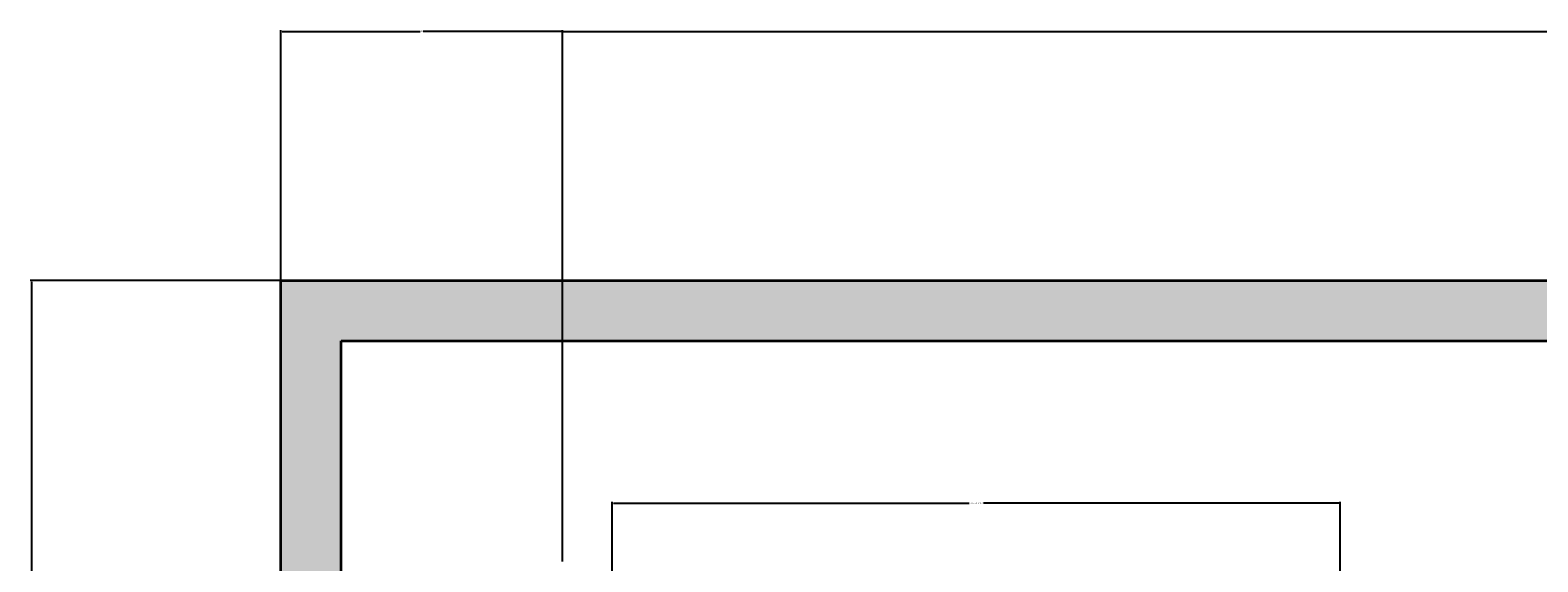
# Model space of a CAD drawing. Units: inches. Extents: x 2701 to 6846, y 811 to 2447.
# Tile 12 of 20: x 2701 to 2926, y 1462 to 1541. Entities that reach past the tile are written whole.
import ezdxf

# ---------------------------------------------------------------- set-up
doc = ezdxf.new("R2010")
doc.units = ezdxf.units.IN
doc.layers.add('A-ANNO-DIMS', color=2, linetype='Continuous', lineweight=18)
doc.layers.add('C-PROP', color=7, linetype='Continuous', lineweight=35)
doc.layers.add('C-PROP-PATT', color=18, linetype='Continuous', lineweight=13, true_color=0x000000)
doc.styles.get("Standard").update_dxf_attribs({"font": 'arial.ttf'})
doc.dimstyles.get("Standard").update_dxf_attribs({"dimtxt": 0.18, "dimasz": 0.18, "dimexe": 0.18, "dimexo": 0.0625, "dimgap": 0.09, "dimtad": 0, "dimtih": 1, "dimtoh": 1, "dimdec": 4, "dimzin": 0, "dimdsep": 46, "dimtxsty": 'Standard', "dimcen": 0.09, "dimadec": 0, "dimazin": 0, "dimtfac": 1, "dimtdec": 4, "dimtofl": 0, "dimtmove": 0, "dimatfit": 3, "dimfxl": 1, "dimtolj": 1, "dimtzin": 0, "dimarcsym": 0})

# ---------------------------------------------------------------- blocks, each defined once
blk = doc.blocks.new('*D49')
at = {"layer": 'A-ANNO-DIMS', "color": 0, "lineweight": -2, "transparency": 16777216}
for p, q in [((2787.42, 1454.59), (2787.42, 1471)), ((2787.6, 1470.82), (2840.65, 1470.82)), ((2895.86, 1470.82), (2842.8, 1470.82)), ((2896.04, 1454.59), (2896.04, 1471))]:
    blk.add_line(p, q, dxfattribs=at)
at = {"layer": 'A-ANNO-DIMS', "color": 0, "transparency": 16777216}
for points in [[(2787.6, 1470.85), (2787.6, 1470.79), (2787.42, 1470.82)], [(2895.86, 1470.85), (2895.86, 1470.79), (2896.04, 1470.82)]]:
    blk.add_solid(points, dxfattribs=at)
at = {"layer": 'Defpoints', "color": 0, "transparency": 16777216}
for p in [(2787.42, 1470.82), (2787.42, 1454.53), (2896.04, 1454.53)]:
    blk.add_point(p, dxfattribs=at)
at = {"layer": 'A-ANNO-DIMS', "color": 0, "transparency": 16777216, "insert": (2841.73, 1470.82), "char_height": 0.18, "attachment_point": 5}
blk.add_mtext('\\A1;BED GROUP 109', dxfattribs=at)
blk = doc.blocks.new('*D66')
at = {"layer": 'A-ANNO-DIMS', "color": 0, "lineweight": -2, "transparency": 16777216}
for p, q in [((2737.91, 1504.05), (2700.59, 1504.05)), ((2700.77, 1503.87), (2700.77, 1180.23)), ((2700.77, 856.23), (2700.77, 1179.87)), ((2737.91, 856.05), (2700.59, 856.05))]:
    blk.add_line(p, q, dxfattribs=at)
at = {"layer": 'A-ANNO-DIMS', "color": 0, "transparency": 16777216}
for points in [[(2700.74, 1503.87), (2700.8, 1503.87), (2700.77, 1504.05)], [(2700.74, 856.23), (2700.8, 856.23), (2700.77, 856.05)]]:
    blk.add_solid(points, dxfattribs=at)
at = {"layer": 'Defpoints', "color": 0, "transparency": 16777216}
for p in [(2700.77, 1504.05), (2737.97, 1504.05), (2737.97, 856.05)]:
    blk.add_point(p, dxfattribs=at)
at = {"layer": 'A-ANNO-DIMS', "color": 0, "transparency": 16777216, "insert": (2700.77, 1180.05), "char_height": 0.18, "attachment_point": 5}
blk.add_mtext('\\A1;648', dxfattribs=at)
blk = doc.blocks.new('*D67')
at = {"layer": 'A-ANNO-DIMS', "color": 0, "lineweight": -2, "transparency": 16777216}
for p, q in [((2779.97, 1462.11), (2779.97, 1541.43)), ((2780.15, 1541.25), (2935.68, 1541.25)), ((3091.79, 1541.25), (2936.26, 1541.25)), ((3091.97, 1462.11), (3091.97, 1541.43))]:
    blk.add_line(p, q, dxfattribs=at)
at = {"layer": 'A-ANNO-DIMS', "color": 0, "transparency": 16777216}
for points in [[(2780.15, 1541.28), (2780.15, 1541.22), (2779.97, 1541.25)], [(3091.79, 1541.28), (3091.79, 1541.22), (3091.97, 1541.25)]]:
    blk.add_solid(points, dxfattribs=at)
at = {"layer": 'Defpoints', "color": 0, "transparency": 16777216}
for p in [(3091.97, 1541.25), (2779.97, 1462.05), (3091.97, 1462.05)]:
    blk.add_point(p, dxfattribs=at)
at = {"layer": 'A-ANNO-DIMS', "color": 0, "transparency": 16777216, "insert": (2935.97, 1541.25), "char_height": 0.18, "attachment_point": 5}
blk.add_mtext('\\A1;312', dxfattribs=at)
blk = doc.blocks.new('*D69')
at = {"layer": 'A-ANNO-DIMS', "color": 0, "lineweight": -2, "transparency": 16777216}
for p, q in [((2737.97, 1504.11), (2737.97, 1541.43)), ((2738.15, 1541.25), (2758.75, 1541.25)), ((2779.79, 1541.25), (2759.19, 1541.25)), ((2779.97, 1462.11), (2779.97, 1541.43))]:
    blk.add_line(p, q, dxfattribs=at)
at = {"layer": 'A-ANNO-DIMS', "color": 0, "transparency": 16777216}
for points in [[(2738.15, 1541.28), (2738.15, 1541.22), (2737.97, 1541.25)], [(2779.79, 1541.28), (2779.79, 1541.22), (2779.97, 1541.25)]]:
    blk.add_solid(points, dxfattribs=at)
at = {"layer": 'Defpoints', "color": 0, "transparency": 16777216}
for p in [(2779.97, 1541.25), (2737.97, 1504.05), (2779.97, 1462.05)]:
    blk.add_point(p, dxfattribs=at)
at = {"layer": 'A-ANNO-DIMS', "color": 0, "transparency": 16777216, "insert": (2758.97, 1541.25), "char_height": 0.18, "attachment_point": 5}
blk.add_mtext('\\A1;42', dxfattribs=at)

msp = doc.modelspace()

# ---------------------------------------------------------------- hatches: boundary and pattern name
at = {"layer": 'C-PROP-PATT'}
h = msp.add_hatch(color=256, dxfattribs=at)
h.dxf.hatch_style = 1
h.paths.add_polyline_path([(3145.97, 1504.05), (2737.97, 1504.05), (2737.97, 967.05), (2746.97, 967.05), (2746.97, 1495.05), (3136.97, 1495.05), (3136.97, 865.05), (3130.97, 865.05), (3130.97, 856.05), (3145.97, 856.05)])
h.paths.add_polyline_path([(3070.97, 865.05), (2746.97, 865.05), (2746.97, 871.05), (2737.97, 871.05), (2737.97, 856.05), (3070.97, 856.05)], flags=17)

# ---------------------------------------------------------------- linework, layer by layer
at = {"layer": 'C-PROP'}
for p, q in [((2737.97, 1504.05), (3145.97, 1504.05)), ((2737.97, 919.05), (2737.97, 1504.05)), ((2746.97, 1495.05), (3136.97, 1495.05)), ((2746.97, 967.05), (2746.97, 1495.05))]:
    msp.add_line(p, q, dxfattribs=at)

# ---------------------------------------------------------------- dimensions: what is measured, and where the dimension line sits
at = {"layer": 'A-ANNO-DIMS'}
for base, p1, p2, picture, middle in [((2779.97, 1541.25), (2737.97, 1504.05), (2779.97, 1462.05), '*D69', (2758.97, 1541.25)), ((3091.97, 1541.25), (2779.97, 1462.05), (3091.97, 1462.05), '*D67', (2935.97, 1541.25))]:
    dim = msp.add_linear_dim(base=base, p1=p1, p2=p2, dimstyle='Standard', override={"dimdec": 0, "dimlfac": 1, "dimrnd": 0, "dimzin": 0, "dimdsep": 46, "dimlunit": 2}, dxfattribs=at)
    dim.commit()
    dim.dimension.update_dxf_attribs({"geometry": picture, "text_midpoint": middle})
dim = msp.add_linear_dim(base=(2700.77, 1504.05), p1=(2737.97, 856.05), p2=(2737.97, 1504.05), angle=90, dimstyle='Standard', override={"dimdec": 0, "dimlfac": 1, "dimrnd": 0, "dimzin": 0, "dimdsep": 46, "dimlunit": 2}, dxfattribs=at)
dim.commit()
dim.dimension.update_dxf_attribs({"geometry": '*D66', "text_midpoint": (2700.77, 1180.05)})
dim = msp.add_linear_dim(base=(2787.42, 1470.82), p1=(2896.04, 1454.53), p2=(2787.42, 1454.53), angle=180, text='BED GROUP <>', dimstyle='Standard', override={"dimdec": 0, "dimlfac": 1, "dimrnd": 0, "dimzin": 0, "dimdsep": 46, "dimlunit": 2}, dxfattribs=at)
dim.commit()
dim.dimension.update_dxf_attribs({"geometry": '*D49', "text_midpoint": (2841.73, 1470.82)})

doc.saveas('drawing.dxf')
